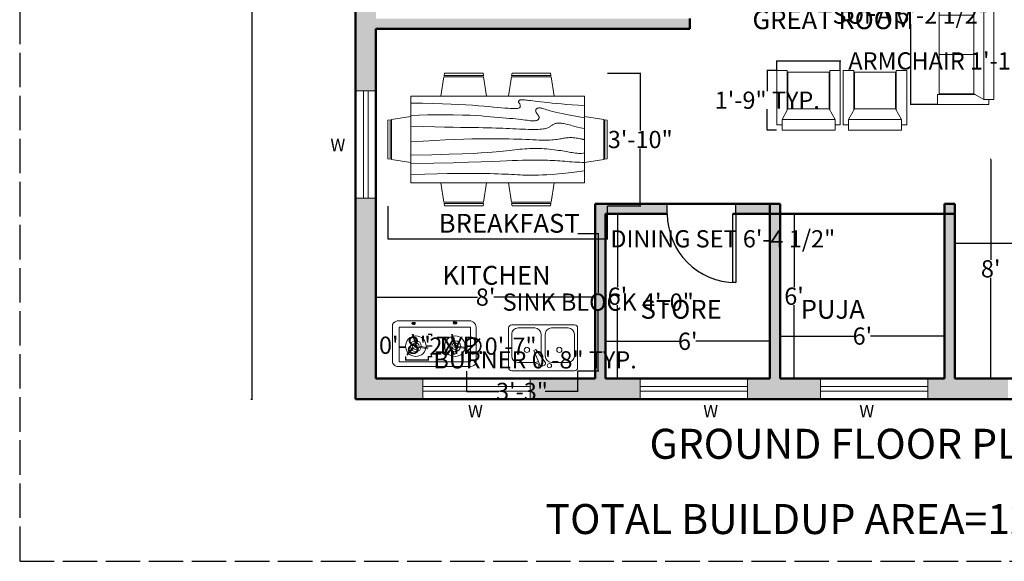
# Model space of a CAD drawing. Units: inches. Extents: x 2905 to 3459, y 4225 to 4672.
# Tile 1 of 3: x 2905 to 3248, y 4225 to 4414. Entities that reach past the tile are written whole.
import ezdxf

# ---------------------------------------------------------------- set-up
doc = ezdxf.new("R2010")
doc.units = ezdxf.units.IN
doc.header["$MEASUREMENT"] = 0
doc.linetypes.add('ACAD_ISO02W100', pattern=[15, 12, -3])
doc.layers.get('0').update_dxf_attribs({"color": 252})
for name, color, linetype, lineweight in [('A-ANNO-DIMS', 2, 'Continuous', 18), ('A-ANNO-TEXT', 7, 'Continuous', 18), ('A-ANNO-TTLB', 7, 'ACAD_ISO02W100', 25), ('A-AREA-IDEN', 7, 'Continuous', 25), ('A-DOOR', 3, 'Continuous', 25), ('A-EQPM', 8, 'Continuous', 18), ('A-FLOR-FIXT', 9, 'Continuous', 18), ('A-GLAZ', 4, 'Continuous', 18), ('A-WALL-PATT', 251, 'Continuous', 13), ('furniture', 8, 'Continuous', 18), ('walls', 251, 'Continuous', 50)]:
    doc.layers.add(name, color=color, linetype=linetype, lineweight=lineweight)
doc.styles.add('ATT', font='TXT')
doc.styles.get("Standard").update_dxf_attribs({"font": 'arial.ttf'})
doc.dimstyles.get("Standard").update_dxf_attribs({"dimtxt": 6, "dimasz": 0.18, "dimexe": 0.18, "dimexo": 0.0625, "dimgap": 0.09, "dimtad": 0, "dimtih": 1, "dimtoh": 1, "dimzin": 0, "dimdsep": 46, "dimlunit": 3, "dimtxsty": 'Standard', "dimcen": 0.09, "dimadec": 0, "dimazin": 0, "dimtfac": 1, "dimtofl": 0, "dimtmove": 0, "dimatfit": 3, "dimfxl": 1, "dimtolj": 1, "dimtzin": 0, "dimarcsym": 0})

# ---------------------------------------------------------------- blocks, each defined once
blk = doc.blocks.new('*U2')
for p, q in [((0, 0), (0, -6)), ((40, 0), (40, -6))]:
    blk.add_line(p, q)
blk.add_lwpolyline([(0, 0), (0, 40), (1.75, 40), (1.75, 0)], close=True)
blk.add_arc((0, 0), 40, 0, 90)
blk = doc.blocks.new('15PSNK10')
at = {"color": 0, "linetype": 'ByBlock'}
for p, q in [((0, 15), (0, -15)), ((20.5, 16.5), (1.5, 16.5)), ((7, 15), (17.5, 15)), ((22, -15), (22, 15)), ((4, 4), (4, 12)), ((20.5, 12), (20.5, 4)), ((2.37, -0.1), (2.77, 0.6)), ((10.18, -3.57), (4.27, 0.87)), ((17.5, 1), (7, 1)), ((2.88, -1.54), (9.68, -4.43)), ((4, -12), (4, -4)), ((7.04, -1), (17.5, -1)), ((9.68, -4.43), (10.18, -3.57)), ((20.5, -4), (20.5, -12)), ((1.5, -16.5), (20.5, -16.5)), ((17.5, -15), (7, -15))]:
    blk.add_line(p, q, dxfattribs=at)
for centre, radius in [((10, 7.75), 1.25), ((2.5, 3), 1), ((2.5, -3), 1), ((10, -7.75), 1.25)]:
    blk.add_circle(centre, radius, dxfattribs=at)
for centre, radius, start, end in [((1.5, 15), 1.5, 90, 180), ((7, 12), 3, 90, 180), ((17.5, 12), 3, 0, 90), ((20.5, 15), 1.5, 0, 90), ((3.63, 0.1), 1, 50.5377, 150), ((7, 4), 3, 180, 270), ((17.5, 4), 3, 270, 0), ((3.23, -0.6), 1, 150, 249.4623), ((7, -4), 3, 146.607, 180), ((17.5, -4), 3, 0, 90), ((7, -12), 3, 180, 270), ((17.5, -12), 3, 270, 0), ((1.5, -15), 1.5, 180, 270), ((20.5, -15), 1.5, 270, 0)]:
    blk.add_arc(centre, radius, start, end, dxfattribs=at)
at = {"color": 0, "linetype": 'ByBlock', "style": 'ATT'}
for tag, p, flags in [('ITEM', (0, -26), 3), ('ROOM_NUMBER', (0, -35), 1)]:
    blk.add_attdef(tag, p, '', height=6, dxfattribs=dict(at, flags=flags))
blk = doc.blocks.new('Dining Set - 36 x 72 in.')
for p, q in [((-22.2343, 26.00059), (-23.4847, 17.99762)), ((-22.2304, 26), (-5.7608, 26)), ((-22, 27.5), (-22.1562, 26.50042)), ((-5.8416, 26.5), (-22.1534, 26.5)), ((-22, 27.5), (-6, 27.5)), ((-5.8437, 26.49966), (-6, 27.5)), ((-4.5152, 17.99762), (-5.7655, 25.99926)), ((5.7657, 26.00059), (4.5153, 17.99762)), ((5.7696, 26), (22.2392, 26)), ((6, 27.5), (5.8438, 26.50042)), ((22.1584, 26.5), (5.8466, 26.5)), ((6, 27.5), (22, 27.5)), ((22.1563, 26.49966), (22, 27.5)), ((23.4848, 17.99762), (22.2345, 25.99926)), ((36, 18), (-36, 18)), ((-36, 18), (-36, -18)), ((36, -18), (36, 18)), ((-44.0006, 8.23428), (-35.9976, 9.48474)), ((-44, 8.23041), (-44, -8.23915)), ((44.0006, 8.23428), (35.9976, 9.48474)), ((44, 8.23041), (44, -8.23915)), ((-45.5, 8), (-44.5004, 8.15617)), ((-45.5, 8), (-45.5, -8)), ((-44.5, -8.15843), (-44.5, 8.15338)), ((44.5, -8.15843), (44.5, 8.15338)), ((45.5, 8), (44.5005, 8.15617)), ((45.5, 8), (45.5, -8)), ((-44.4997, -8.15631), (-45.5, -8)), ((44.4997, -8.15631), (45.5, -8)), ((-35.9976, -9.48476), (-43.9993, -8.2345)), ((35.9976, -9.48476), (43.9993, -8.2345)), ((-36, -18), (36, -18)), ((-22.2343, -26.0006), (-23.4847, -17.99762)), ((-4.5152, -17.99762), (-5.7655, -25.99928)), ((5.7657, -26.0006), (4.5153, -17.99762)), ((23.4848, -17.99762), (22.2345, -25.99928)), ((-22.2304, -26), (-5.7608, -26)), ((-22, -27.5), (-22.1562, -26.50044)), ((-5.8416, -26.5), (-22.1534, -26.5)), ((-22, -27.5), (-6, -27.5)), ((-5.8437, -26.49967), (-6, -27.5)), ((5.7696, -26), (22.2392, -26)), ((6, -27.5), (5.8438, -26.50044)), ((22.1584, -26.5), (5.8466, -26.5)), ((6, -27.5), (22, -27.5)), ((22.1563, -26.49967), (22, -27.5))]:
    blk.add_line(p, q)
for points in [[(-36, 15), (-31.1772, 14.97754), (-26.8079, 14.91406), (-22.8538, 14.81543), (-19.276, 14.6875), (-16.0362, 14.53613), (-13.0957, 14.36718), (-10.4159, 14.18652), (-7.9583, 14), (-5.6904, 13.81315), (-3.6035, 13.63021), (-1.6954, 13.45508), (0.0365, 13.29166), (1.5945, 13.14388), (2.9811, 13.01562), (4.1988, 12.9108), (5.25, 12.83333), (6.1393, 12.78613), (6.8802, 12.76823), (7.4883, 12.77767), (7.9792, 12.8125), (8.3685, 12.87077), (8.6719, 12.95052), (8.9049, 13.0498), (9.0833, 13.16666), (9.2205, 13.29899), (9.3216, 13.44401), (9.3895, 13.59879), (9.4271, 13.76041), (9.4373, 13.92594), (9.4232, 14.09245), (9.3875, 14.257), (9.3333, 14.41666), (9.2638, 14.56917), (9.1836, 14.71484), (9.0975, 14.85465), (9.0104, 14.98958), (8.9272, 15.1206), (8.8529, 15.2487), (8.7922, 15.37483), (8.75, 15.5), (8.7305, 15.62467), (8.7344, 15.74739), (8.7617, 15.86621), (8.8125, 15.97916), (8.8867, 16.08431), (8.9844, 16.17968), (9.1055, 16.26334), (9.25, 16.33333), (9.4189, 16.38802), (9.6172, 16.42708), (9.8506, 16.45052), (10.125, 16.45833), (10.4463, 16.45052), (10.8203, 16.42708), (11.2529, 16.38802), (11.75, 16.33333), (12.3184, 16.26318), (12.9694, 16.17838), (13.7151, 16.07991), (14.5677, 15.96875), (15.5395, 15.84586), (16.6426, 15.71224), (17.8893, 15.56884), (19.2917, 15.41666), (20.859, 15.25667), (22.5879, 15.08984), (24.4721, 14.91715), (26.5052, 14.73958), (28.6809, 14.5581), (30.9929, 14.3737), (33.4347, 14.18733), (36, 14)], [(-36, 10), (-28.9766, 10.14274), (-23.1725, 10.20442), (-18.4241, 10.19775), (-14.5677, 10.13541), (-11.4399, 10.03011), (-8.877, 9.89453), (-6.7154, 9.74137), (-4.7917, 9.58333), (-2.9698, 9.43082), (-1.2246, 9.28515), (0.4415, 9.14534), (2.026, 9.01041), (3.5266, 8.87939), (4.9408, 8.7513), (6.266, 8.62516), (7.5, 8.5), (8.6411, 8.37549), (9.6914, 8.2539), (10.6538, 8.13818), (11.5312, 8.03125), (12.3267, 7.93603), (13.043, 7.85547), (13.6831, 7.79248), (14.25, 7.75), (14.7471, 7.7303), (15.1797, 7.73307), (15.5537, 7.75732), (15.875, 7.80208), (16.1494, 7.86637), (16.3828, 7.94922), (16.5811, 8.04964), (16.75, 8.16666), (16.8944, 8.29915), (17.0143, 8.44531), (17.1089, 8.60319), (17.1771, 8.77083), (17.218, 8.94629), (17.2305, 9.1276), (17.2137, 9.31282), (17.1667, 9.5), (17.0895, 9.6875), (16.987, 9.875), (16.8649, 10.0625), (16.7292, 10.25), (16.5856, 10.4375), (16.4401, 10.625), (16.2985, 10.8125), (16.1667, 11), (16.05, 11.18733), (15.9518, 11.3737), (15.8752, 11.5581), (15.8229, 11.73958), (15.798, 11.91715), (15.8034, 12.08984), (15.842, 12.25667), (15.9167, 12.41666), (16.0295, 12.56836), (16.1784, 12.70833), (16.3605, 12.83268), (16.5729, 12.9375), (16.8127, 13.01888), (17.0768, 13.07291), (17.3625, 13.0957), (17.6667, 13.08333), (17.9894, 13.03312), (18.3418, 12.94726), (18.7382, 12.82918), (19.1927, 12.68229), (19.7195, 12.51001), (20.3327, 12.31575), (21.0465, 12.10294), (21.875, 11.875), (22.8357, 11.63354), (23.959, 11.37304), (25.2786, 11.08618), (26.8282, 10.76562), (28.6414, 10.40405), (30.752, 9.99414), (33.1936, 9.52856), (36, 9)], [(-36, 5.5), (-30.7157, 5.3348), (-26.069, 5.20963), (-21.9946, 5.11767), (-18.4271, 5.05208), (-15.3009, 5.00602), (-12.5508, 4.97265), (-10.1112, 4.94515), (-7.9167, 4.91666), (-5.909, 4.88167), (-4.0586, 4.83984), (-2.3429, 4.79215), (-0.7396, 4.73958), (0.7739, 4.6831), (2.22, 4.6237), (3.6213, 4.56233), (5, 4.5), (6.373, 4.43782), (7.7344, 4.3776), (9.0723, 4.32129), (10.375, 4.27083), (11.6309, 4.22819), (12.8281, 4.19531), (13.9551, 4.17415), (15, 4.16666), (15.954, 4.17448), (16.819, 4.19791), (17.6001, 4.23698), (18.3021, 4.29166), (18.9299, 4.36198), (19.4883, 4.44791), (19.9823, 4.54948), (20.4167, 4.66666), (20.7969, 4.79899), (21.1302, 4.94401), (21.4245, 5.09879), (21.6875, 5.26041), (21.9271, 5.42594), (22.1511, 5.59245), (22.3672, 5.757), (22.5834, 5.91666), (22.8065, 6.06868), (23.0404, 6.21093), (23.2879, 6.34147), (23.5521, 6.45833), (23.8358, 6.55957), (24.142, 6.64323), (24.4735, 6.70735), (24.8334, 6.75), (25.2235, 6.76969), (25.642, 6.76692), (26.0858, 6.74267), (26.5521, 6.69791), (27.0379, 6.63362), (27.5404, 6.55078), (28.0565, 6.45036), (28.5834, 6.33333), (29.1242, 6.19987), (29.7071, 6.04687), (30.3661, 5.87044), (31.1354, 5.66666), (32.0493, 5.43164), (33.142, 5.16146), (34.4475, 4.85221), (36, 4.5)], [(-36, -1), (-30.7915, -0.6591), (-26.0195, -0.38216), (-21.6519, -0.16284), (-17.6563, 0.00521), (-14.0005, 0.12833), (-10.6523, 0.21289), (-7.5796, 0.26522), (-4.75, 0.29166), (-2.134, 0.29793), (0.2878, 0.28711), (2.5317, 0.26163), (4.6146, 0.22396), (6.5529, 0.17651), (8.3633, 0.12174), (10.0623, 0.06209), (11.6667, 0), (13.1899, -0.06201), (14.6341, -0.1211), (15.9982, -0.17432), (17.2813, -0.21875), (18.4823, -0.25147), (19.6003, -0.26953), (20.6343, -0.27002), (21.5834, -0.25), (22.4481, -0.20768), (23.2357, -0.14584), (23.9549, -0.06836), (24.6146, 0.02083), (25.2235, 0.11784), (25.7904, 0.21875), (26.3241, 0.31966), (26.8334, 0.41666), (27.3265, 0.50618), (27.8099, 0.58593), (28.2894, 0.65397), (28.7709, 0.70833), (29.2601, 0.74707), (29.763, 0.76823), (30.2855, 0.76985), (30.8334, 0.75), (31.4088, 0.70784), (31.9994, 0.64713), (32.589, 0.57275), (33.1615, 0.48958), (33.7008, 0.4025), (34.1908, 0.3164), (34.6153, 0.23616), (34.9584, 0.16666), (35.2099, 0.11165), (35.3848, 0.07031), (35.504, 0.04069), (35.5886, 0.02083), (35.6594, 0.00879), (35.7377, 0.0026), (35.8442, 0.00032), (36, 0)], [(-36, -6.5), (-27.1843, -6.31267), (-20.084, -6.1263), (-14.469, -5.9419), (-10.1094, -5.76042), (-6.7752, -5.58285), (-4.2363, -5.41016), (-2.2629, -5.24333), (-0.625, -5.08334), (0.8708, -4.93099), (2.2715, -4.78646), (3.5872, -4.64974), (4.8281, -4.52084), (6.0046, -4.39974), (7.127, -4.28646), (8.2053, -4.18099), (9.25, -4.08334), (10.2705, -3.99382), (11.2734, -3.91407), (12.2647, -3.84603), (13.25, -3.79167), (14.2354, -3.75293), (15.2266, -3.73177), (16.2295, -3.73015), (17.25, -3.75), (18.2912, -3.79248), (19.3451, -3.85547), (20.4009, -3.93604), (21.4479, -4.03125), (22.4754, -4.13819), (23.4727, -4.25391), (24.4289, -4.37549), (25.3334, -4.5), (26.1785, -4.62492), (26.9694, -4.74935), (27.7145, -4.87281), (28.4219, -4.99479), (29.1, -5.11483), (29.7572, -5.23242), (30.4016, -5.34709), (31.0417, -5.45834), (31.6837, -5.56437), (32.3262, -5.65821), (32.9658, -5.73153), (33.599, -5.77604), (34.2224, -5.78345), (34.8327, -5.74545), (35.4264, -5.65373), (36, -5.5)], [(-36, -10), (-26.4022, -9.81299), (-18.4675, -9.62891), (-11.9839, -9.45069), (-6.7396, -9.28125), (-2.5226, -9.12354), (0.8789, -8.98047), (3.6769, -8.85498), (6.0833, -8.75), (8.2767, -8.66765), (10.3021, -8.60677), (12.1712, -8.56543), (13.8958, -8.54167), (15.4876, -8.53353), (16.9583, -8.53907), (18.3197, -8.55632), (19.5834, -8.58334), (20.7616, -8.61841), (21.8685, -8.66081), (22.9188, -8.71004), (23.9271, -8.76563), (24.9081, -8.82707), (25.8763, -8.89388), (26.8465, -8.96558), (27.8334, -9.04167), (28.8474, -9.12118), (29.8828, -9.20117), (30.93, -9.27824), (31.9792, -9.34896), (33.0205, -9.40991), (34.0443, -9.45768), (35.0407, -9.48885), (36, -9.5)], [(-36, -14.5), (-30.0881, -14.33513), (-25.0332, -14.21224), (-20.7312, -14.12647), (-17.0781, -14.07292), (-13.97, -14.04671), (-11.3027, -14.04297), (-8.9724, -14.05681), (-6.875, -14.08334), (-4.9224, -14.11833), (-3.0905, -14.16016), (-1.3709, -14.20785), (0.2448, -14.26042), (1.7647, -14.3169), (3.1973, -14.3763), (4.5507, -14.43767), (5.8333, -14.5), (7.0554, -14.5621), (8.235, -14.62175), (9.3922, -14.67652), (10.5469, -14.72396), (11.7192, -14.76164), (12.929, -14.78711), (14.1965, -14.79794), (15.5417, -14.79167), (16.9933, -14.76424), (18.6152, -14.70508), (20.4804, -14.60197), (22.6615, -14.44271), (25.2312, -14.21509), (28.2624, -13.9069), (31.8277, -13.50594), (36, -13)]]:
    blk.add_lwpolyline(points)
blk = doc.blocks.new('FABRIC SOFA 4S')
at = {"layer": 'furniture'}
for p, q in [((3, 54), (34, 54)), ((3, 51), (3, 54)), ((34, 48), (34, 54)), ((0, -51), (0, 51)), ((6, 51), (0, 51)), ((6, -51), (6, 51)), ((12, 47.63), (6, 51)), ((11.14, 48), (34, 48)), ((33, 23.81), (12, 23.81)), ((33, 0), (12, 0)), ((33, -23.81), (12, -23.81)), ((6, -51), (0, -51)), ((3, -54), (3, -51)), ((6, -51), (12, -47.63)), ((11.54, -48), (34, -48)), ((34, -48), (34, -54)), ((3, -54), (34, -54))]:
    blk.add_line(p, q, dxfattribs=at)
blk.add_lwpolyline([(12, -47.63), (12, 47.63), (33, 47.63), (33, -47.63)], close=True, dxfattribs=at)
blk = doc.blocks.new('FABRIC SOFA 1S')
at = {"layer": 'furniture'}
for p, q in [((3, 18.12), (34, 18.12)), ((3, 15.12), (3, 18.12)), ((34, 12.12), (34, 18.12)), ((0, -15.12), (0, 15.12)), ((6, 15.12), (0, 15.12)), ((6, -15.12), (6, 15.12)), ((12, 11.75), (6, 15.12)), ((11.33, 12.12), (34, 12.12)), ((6, -15.12), (0, -15.12)), ((3, -18.12), (3, -15.12)), ((6, -15.12), (12, -11.75)), ((11.33, -12.12), (34, -12.12)), ((34, -12.12), (34, -18.12)), ((3, -18.12), (34, -18.12))]:
    blk.add_line(p, q, dxfattribs=at)
blk.add_lwpolyline([(12, -11.75), (12, 11.75), (33, 11.75), (33, -11.75)], close=True, dxfattribs=at)
blk = doc.blocks.new('*D17')
at = {"layer": 'A-ANNO-DIMS', "color": 0, "lineweight": -2, "transparency": 16777216}
for p, q in [((3243.15, 4365.3), (3243.03, 4365.3)), ((3243.21, 4365.12), (3243.21, 4330.25)), ((3243.21, 4289.08), (3243.21, 4323.95)), ((3243.03, 4288.9), (3243.39, 4288.9))]:
    blk.add_line(p, q, dxfattribs=at)
at = {"layer": 'A-ANNO-DIMS', "color": 0, "transparency": 16777216}
for points in [[(3243.18, 4365.12), (3243.24, 4365.12), (3243.21, 4365.3)], [(3243.18, 4289.08), (3243.24, 4289.08), (3243.21, 4288.9)]]:
    blk.add_solid(points, dxfattribs=at)
at = {"layer": 'Defpoints', "color": 0, "transparency": 16777216}
for p in [(3243.21, 4365.3), (3243.21, 4365.3), (3242.97, 4288.9)]:
    blk.add_point(p, dxfattribs=at)
at = {"layer": 'A-ANNO-DIMS', "color": 0, "transparency": 16777216, "insert": (3243.21, 4327.1), "char_height": 6, "attachment_point": 5}
blk.add_mtext("\\A1;8'", dxfattribs=at)
blk = doc.blocks.new('*D18')
at = {"layer": 'A-ANNO-DIMS', "color": 0, "lineweight": -2, "transparency": 16777216}
for p, q in [((3230.73, 4336.07), (3230.73, 4336.19)), ((3230.91, 4336.01), (3284.92, 4336.01)), ((3348.73, 4336.01), (3294.72, 4336.01)), ((3348.91, 4336.07), (3348.91, 4336.19))]:
    blk.add_line(p, q, dxfattribs=at)
at = {"layer": 'A-ANNO-DIMS', "color": 0, "transparency": 16777216}
for points in [[(3230.91, 4336.04), (3230.91, 4335.98), (3230.73, 4336.01)], [(3348.73, 4336.04), (3348.73, 4335.98), (3348.91, 4336.01)]]:
    blk.add_solid(points, dxfattribs=at)
at = {"layer": 'Defpoints', "color": 0, "transparency": 16777216}
for p in [(3230.73, 4336.01), (3348.91, 4336.01), (3348.91, 4336.01)]:
    blk.add_point(p, dxfattribs=at)
at = {"layer": 'A-ANNO-DIMS', "color": 0, "transparency": 16777216, "insert": (3289.82, 4336.01), "char_height": 6, "attachment_point": 5}
blk.add_mtext("\\A1;12'", dxfattribs=at)
blk = doc.blocks.new('*D19')
at = {"layer": 'A-ANNO-DIMS', "color": 0, "lineweight": -2, "transparency": 16777216}
for p, q in [((3174.67, 4346.02), (3174.67, 4320.7)), ((3174.73, 4346.2), (3174.85, 4346.2)), ((3174.67, 4289.08), (3174.67, 4314.4)), ((3174.73, 4288.9), (3174.85, 4288.9))]:
    blk.add_line(p, q, dxfattribs=at)
at = {"layer": 'A-ANNO-DIMS', "color": 0, "transparency": 16777216}
for points in [[(3174.64, 4346.02), (3174.7, 4346.02), (3174.67, 4346.2)], [(3174.64, 4289.08), (3174.7, 4289.08), (3174.67, 4288.9)]]:
    blk.add_solid(points, dxfattribs=at)
at = {"layer": 'Defpoints', "color": 0, "transparency": 16777216}
for p in [(3174.67, 4346.2), (3174.67, 4288.9), (3174.67, 4288.9)]:
    blk.add_point(p, dxfattribs=at)
at = {"layer": 'A-ANNO-DIMS', "color": 0, "transparency": 16777216, "insert": (3174.67, 4317.55), "char_height": 6, "attachment_point": 5}
blk.add_mtext("\\A1;6'", dxfattribs=at)
blk = doc.blocks.new('*D20')
at = {"layer": 'A-ANNO-DIMS', "color": 0, "lineweight": -2, "transparency": 16777216}
for p, q in [((3169.85, 4303.75), (3169.85, 4303.86)), ((3170.03, 4303.68), (3195.63, 4303.68)), ((3226.97, 4303.68), (3201.37, 4303.68)), ((3227.15, 4303.75), (3227.15, 4303.86))]:
    blk.add_line(p, q, dxfattribs=at)
at = {"layer": 'A-ANNO-DIMS', "color": 0, "transparency": 16777216}
for points in [[(3170.03, 4303.71), (3170.03, 4303.65), (3169.85, 4303.68)], [(3226.97, 4303.71), (3226.97, 4303.65), (3227.15, 4303.68)]]:
    blk.add_solid(points, dxfattribs=at)
at = {"layer": 'Defpoints', "color": 0, "transparency": 16777216}
for p in [(3169.85, 4303.68), (3227.15, 4303.68), (3227.15, 4303.68)]:
    blk.add_point(p, dxfattribs=at)
at = {"layer": 'A-ANNO-DIMS', "color": 0, "transparency": 16777216, "insert": (3198.5, 4303.68), "char_height": 6, "attachment_point": 5}
blk.add_mtext("\\A1;6'", dxfattribs=at)
blk = doc.blocks.new('*D21')
at = {"layer": 'A-ANNO-DIMS', "color": 0, "lineweight": -2, "transparency": 16777216}
for p, q in [((3113.13, 4346.02), (3113.13, 4320.7)), ((3113.19, 4346.2), (3113.31, 4346.2)), ((3113.13, 4289.08), (3113.13, 4314.4)), ((3113.19, 4288.9), (3113.31, 4288.9))]:
    blk.add_line(p, q, dxfattribs=at)
at = {"layer": 'A-ANNO-DIMS', "color": 0, "transparency": 16777216}
for points in [[(3113.1, 4346.02), (3113.16, 4346.02), (3113.13, 4346.2)], [(3113.1, 4289.08), (3113.16, 4289.08), (3113.13, 4288.9)]]:
    blk.add_solid(points, dxfattribs=at)
at = {"layer": 'Defpoints', "color": 0, "transparency": 16777216}
for p in [(3113.13, 4346.2), (3113.13, 4288.9), (3113.13, 4288.9)]:
    blk.add_point(p, dxfattribs=at)
at = {"layer": 'A-ANNO-DIMS', "color": 0, "transparency": 16777216, "insert": (3113.13, 4317.55), "char_height": 6, "attachment_point": 5}
blk.add_mtext("\\A1;6'", dxfattribs=at)
blk = doc.blocks.new('*D22')
at = {"layer": 'A-ANNO-DIMS', "color": 0, "lineweight": -2, "transparency": 16777216}
for p, q in [((3108.97, 4301.79), (3108.97, 4301.68)), ((3109.15, 4301.86), (3134.75, 4301.86)), ((3166.09, 4301.86), (3140.48, 4301.86)), ((3166.27, 4301.92), (3166.27, 4302.04))]:
    blk.add_line(p, q, dxfattribs=at)
at = {"layer": 'A-ANNO-DIMS', "color": 0, "transparency": 16777216}
for points in [[(3109.15, 4301.89), (3109.15, 4301.83), (3108.97, 4301.86)], [(3166.09, 4301.89), (3166.09, 4301.83), (3166.27, 4301.86)]]:
    blk.add_solid(points, dxfattribs=at)
at = {"layer": 'Defpoints', "color": 0, "transparency": 16777216}
for p in [(3108.97, 4301.86), (3166.27, 4301.86), (3166.27, 4301.86)]:
    blk.add_point(p, dxfattribs=at)
at = {"layer": 'A-ANNO-DIMS', "color": 0, "transparency": 16777216, "insert": (3137.62, 4301.86), "char_height": 6, "attachment_point": 5}
blk.add_mtext("\\A1;6'", dxfattribs=at)
blk = doc.blocks.new('*D24')
at = {"layer": 'A-ANNO-DIMS', "color": 0, "lineweight": -2, "transparency": 16777216}
for p, q in [((3028.98, 4317.18), (3028.98, 4317.07)), ((3029.16, 4317.25), (3064.33, 4317.25)), ((3105.21, 4317.25), (3070.04, 4317.25)), ((3105.39, 4317.18), (3105.39, 4317.07))]:
    blk.add_line(p, q, dxfattribs=at)
at = {"layer": 'A-ANNO-DIMS', "color": 0, "transparency": 16777216}
for points in [[(3029.16, 4317.28), (3029.16, 4317.22), (3028.98, 4317.25)], [(3105.21, 4317.28), (3105.21, 4317.22), (3105.39, 4317.25)]]:
    blk.add_solid(points, dxfattribs=at)
at = {"layer": 'Defpoints', "color": 0, "transparency": 16777216}
for p in [(3028.98, 4317.25), (3105.39, 4317.25), (3105.39, 4317.25)]:
    blk.add_point(p, dxfattribs=at)
at = {"layer": 'A-ANNO-DIMS', "color": 0, "transparency": 16777216, "insert": (3067.19, 4317.25), "char_height": 6, "attachment_point": 5}
blk.add_mtext("\\A1;8'", dxfattribs=at)
blk = doc.blocks.new('*D25')
at = {"layer": 'A-ANNO-DIMS', "color": 0, "lineweight": -2, "transparency": 16777216}
for p, q in [((2985.39, 4615.99), (2985.98, 4615.99)), ((2985.8, 4615.81), (2985.8, 4452.02)), ((2985.8, 4281.92), (2985.8, 4445.71)), ((2985.39, 4281.74), (2985.98, 4281.74))]:
    blk.add_line(p, q, dxfattribs=at)
at = {"layer": 'A-ANNO-DIMS', "color": 0, "transparency": 16777216}
for points in [[(2985.77, 4615.81), (2985.83, 4615.81), (2985.8, 4615.99)], [(2985.77, 4281.92), (2985.83, 4281.92), (2985.8, 4281.74)]]:
    blk.add_solid(points, dxfattribs=at)
at = {"layer": 'Defpoints', "color": 0, "transparency": 16777216}
for p in [(2985.32, 4615.99), (2985.32, 4281.74), (2985.8, 4281.74)]:
    blk.add_point(p, dxfattribs=at)
at = {"layer": 'A-ANNO-DIMS', "color": 0, "transparency": 16777216, "insert": (2985.8, 4448.86), "char_height": 6, "attachment_point": 5}
blk.add_mtext("\\A1;35'", dxfattribs=at)
blk = doc.blocks.new('WIN-PLAN-STANDARD')
for p, q in [((0, 7.16), (0, 0)), ((37.45, 7.16), (0, 7.16)), ((0, 7.16), (0, 4.38)), ((37.45, 0), (37.45, 7.16)), ((0, 4.38), (37.45, 4.38)), ((37.45, 4.38), (37.45, 2.7)), ((0, 2.7), (37.45, 2.7)), ((0, 0), (37.45, 0))]:
    blk.add_line(p, q)
blk = doc.blocks.new('COOKTOP-BURNER')
for p, q in [((3.4, 4.69), (2.36, 7.73)), ((3.74, 4.7), (2.62, 7.81)), ((4.71, 3.58), (7.87, 2.96)), ((2.54, 3.16), (0.4, 0.64)), ((2.72, 2.87), (0.61, 0.45)), ((4.55, 3.29), (7.8, 2.69))]:
    blk.add_line(p, q)
for radius in [3.58, 1.91, 1.12, 0.464]:
    blk.add_circle((3.58, 3.58), radius)
blk = doc.blocks.new('*D32')
at = {"layer": 'A-ANNO-DIMS', "color": 0, "lineweight": -2, "transparency": 16777216}
for p, q in [((3168.67, 4396.25), (3168.67, 4399.69)), ((3168.85, 4399.51), (3190.61, 4399.51)), ((3190.79, 4396.25), (3190.79, 4399.69)), ((3190.79, 4399.51), (3190.97, 4399.51))]:
    blk.add_line(p, q, dxfattribs=at)
at = {"layer": 'A-ANNO-DIMS', "color": 0, "transparency": 16777216}
for points in [[(3168.85, 4399.54), (3168.85, 4399.48), (3168.67, 4399.51)], [(3190.61, 4399.54), (3190.61, 4399.48), (3190.79, 4399.51)]]:
    blk.add_solid(points, dxfattribs=at)
at = {"layer": 'Defpoints', "color": 0, "transparency": 16777216}
for p in [(3190.79, 4399.51), (3168.67, 4396.19), (3190.79, 4396.19)]:
    blk.add_point(p, dxfattribs=at)
at = {"layer": 'A-ANNO-DIMS', "color": 0, "transparency": 16777216, "insert": (3235.37, 4399.51), "char_height": 6, "attachment_point": 5}
blk.add_mtext('\\A1;ARMCHAIR 1\'-10" TYP.', dxfattribs=at)
blk = doc.blocks.new('*D33')
at = {"layer": 'A-ANNO-DIMS', "color": 0, "lineweight": -2, "transparency": 16777216}
for p, q in [((3168.6, 4396.19), (3165.17, 4396.19)), ((3165.35, 4396.01), (3165.35, 4388.97)), ((3165.35, 4375.62), (3165.35, 4382.66)), ((3168.6, 4375.44), (3165.17, 4375.44))]:
    blk.add_line(p, q, dxfattribs=at)
at = {"layer": 'A-ANNO-DIMS', "color": 0, "transparency": 16777216}
for points in [[(3165.32, 4396.01), (3165.38, 4396.01), (3165.35, 4396.19)], [(3165.32, 4375.62), (3165.38, 4375.62), (3165.35, 4375.44)]]:
    blk.add_solid(points, dxfattribs=at)
at = {"layer": 'Defpoints', "color": 0, "transparency": 16777216}
for p in [(3165.35, 4396.19), (3168.67, 4396.19), (3168.67, 4375.44)]:
    blk.add_point(p, dxfattribs=at)
at = {"layer": 'A-ANNO-DIMS', "color": 0, "transparency": 16777216, "insert": (3165.35, 4385.82), "char_height": 6, "attachment_point": 5}
blk.add_mtext('\\A1;1\'-9" TYP.', dxfattribs=at)
blk = doc.blocks.new('*D38')
at = {"layer": 'A-ANNO-DIMS', "color": 0, "lineweight": -2, "transparency": 16777216}
for p, q in [((3039.29, 4296.52), (3039.29, 4295.22)), ((3047.16, 4296.52), (3047.16, 4295.22)), ((3039.47, 4295.4), (3046.98, 4295.4)), ((3047.16, 4295.4), (3047.34, 4295.4))]:
    blk.add_line(p, q, dxfattribs=at)
at = {"layer": 'A-ANNO-DIMS', "color": 0, "transparency": 16777216}
for points in [[(3039.47, 4295.43), (3039.47, 4295.37), (3039.29, 4295.4)], [(3046.98, 4295.43), (3046.98, 4295.37), (3047.16, 4295.4)]]:
    blk.add_solid(points, dxfattribs=at)
at = {"layer": 'Defpoints', "color": 0, "transparency": 16777216}
for p in [(3039.29, 4296.58), (3047.16, 4296.58), (3047.16, 4295.4)]:
    blk.add_point(p, dxfattribs=at)
at = {"layer": 'A-ANNO-DIMS', "color": 0, "transparency": 16777216, "insert": (3084.44, 4295.4), "char_height": 6, "attachment_point": 5}
blk.add_mtext('\\A1;BURNER 0\'-8" TYP.', dxfattribs=at)
blk = doc.blocks.new('*D39')
at = {"layer": 'A-ANNO-DIMS', "color": 0, "lineweight": -2, "transparency": 16777216}
for p, q in [((3047.22, 4304.39), (3048.52, 4304.39)), ((3048.34, 4304.21), (3048.34, 4303.64)), ((3047.22, 4296.58), (3048.52, 4296.58)), ((3048.34, 4296.76), (3048.34, 4297.33))]:
    blk.add_line(p, q, dxfattribs=at)
at = {"layer": 'A-ANNO-DIMS', "color": 0, "transparency": 16777216}
for points in [[(3048.31, 4304.21), (3048.37, 4304.21), (3048.34, 4304.39)], [(3048.31, 4296.76), (3048.37, 4296.76), (3048.34, 4296.58)]]:
    blk.add_solid(points, dxfattribs=at)
at = {"layer": 'Defpoints', "color": 0, "transparency": 16777216}
for p in [(3047.16, 4304.39), (3048.34, 4304.39), (3047.16, 4296.58)]:
    blk.add_point(p, dxfattribs=at)
at = {"layer": 'A-ANNO-DIMS', "color": 0, "transparency": 16777216, "insert": (3048.34, 4300.48), "char_height": 6, "attachment_point": 5}
blk.add_mtext('\\A1;0\'-8" TYP.', dxfattribs=at)
blk = doc.blocks.new('*D40')
at = {"layer": 'A-ANNO-DIMS', "color": 0, "lineweight": -2, "transparency": 16777216}
for p, q in [((3099.32, 4339.45), (3106.62, 4339.45)), ((3106.44, 4339.27), (3106.44, 4318.71)), ((3106.44, 4291.75), (3106.44, 4312.32)), ((3099.32, 4291.57), (3106.62, 4291.57))]:
    blk.add_line(p, q, dxfattribs=at)
at = {"layer": 'A-ANNO-DIMS', "color": 0, "transparency": 16777216}
for points in [[(3106.41, 4339.27), (3106.47, 4339.27), (3106.44, 4339.45)], [(3106.41, 4291.75), (3106.47, 4291.75), (3106.44, 4291.57)]]:
    blk.add_solid(points, dxfattribs=at)
at = {"layer": 'Defpoints', "color": 0, "transparency": 16777216}
for p in [(3099.26, 4339.45), (3106.44, 4339.45), (3099.26, 4291.57)]:
    blk.add_point(p, dxfattribs=at)
at = {"layer": 'A-ANNO-DIMS', "color": 0, "transparency": 16777216, "insert": (3106.44, 4315.51), "char_height": 6, "attachment_point": 5}
blk.add_mtext('\\A1;SINK BLOCK 4\'-0"', dxfattribs=at)
blk = doc.blocks.new('*D41')
at = {"layer": 'A-ANNO-DIMS', "color": 0, "lineweight": -2, "transparency": 16777216}
for p, q in [((3060.5, 4291.51), (3060.5, 4284.21)), ((3099.26, 4291.51), (3099.26, 4284.21)), ((3060.68, 4284.39), (3071.82, 4284.39)), ((3099.08, 4284.39), (3087.94, 4284.39))]:
    blk.add_line(p, q, dxfattribs=at)
at = {"layer": 'A-ANNO-DIMS', "color": 0, "transparency": 16777216}
for points in [[(3060.68, 4284.42), (3060.68, 4284.36), (3060.5, 4284.39)], [(3099.08, 4284.42), (3099.08, 4284.36), (3099.26, 4284.39)]]:
    blk.add_solid(points, dxfattribs=at)
at = {"layer": 'Defpoints', "color": 0, "transparency": 16777216}
for p in [(3060.5, 4291.57), (3099.26, 4291.57), (3099.26, 4284.39)]:
    blk.add_point(p, dxfattribs=at)
at = {"layer": 'A-ANNO-DIMS', "color": 0, "transparency": 16777216, "insert": (3079.88, 4284.39), "char_height": 6, "attachment_point": 5}
blk.add_mtext('\\A1;3\'-3"', dxfattribs=at)
blk = doc.blocks.new('*D42')
at = {"layer": 'A-ANNO-DIMS', "color": 0, "lineweight": -2, "transparency": 16777216}
for p, q in [((3033.11, 4348.97), (3033.11, 4337.37)), ((3109.6, 4348.97), (3109.6, 4337.37)), ((3033.29, 4337.55), (3109.42, 4337.55)), ((3109.6, 4337.55), (3109.78, 4337.55))]:
    blk.add_line(p, q, dxfattribs=at)
at = {"layer": 'A-ANNO-DIMS', "color": 0, "transparency": 16777216}
for points in [[(3033.29, 4337.58), (3033.29, 4337.52), (3033.11, 4337.55)], [(3109.42, 4337.58), (3109.42, 4337.52), (3109.6, 4337.55)]]:
    blk.add_solid(points, dxfattribs=at)
at = {"layer": 'Defpoints', "color": 0, "transparency": 16777216}
for p in [(3033.11, 4349.03), (3109.6, 4349.03), (3109.6, 4337.55)]:
    blk.add_point(p, dxfattribs=at)
at = {"layer": 'A-ANNO-DIMS', "color": 0, "transparency": 16777216, "insert": (3149.84, 4337.55), "char_height": 6, "attachment_point": 5}
blk.add_mtext('\\A1;DINING SET 6\'-4 1/2"', dxfattribs=at)
blk = doc.blocks.new('*D43')
at = {"layer": 'A-ANNO-DIMS', "color": 0, "lineweight": -2, "transparency": 16777216}
for p, q in [((3109.66, 4395.26), (3121.26, 4395.26)), ((3121.08, 4395.08), (3121.08, 4375.3)), ((3121.08, 4349.21), (3121.08, 4368.99)), ((3109.66, 4349.03), (3121.26, 4349.03))]:
    blk.add_line(p, q, dxfattribs=at)
at = {"layer": 'A-ANNO-DIMS', "color": 0, "transparency": 16777216}
for points in [[(3121.05, 4395.08), (3121.11, 4395.08), (3121.08, 4395.26)], [(3121.05, 4349.21), (3121.11, 4349.21), (3121.08, 4349.03)]]:
    blk.add_solid(points, dxfattribs=at)
at = {"layer": 'Defpoints', "color": 0, "transparency": 16777216}
for p in [(3109.6, 4395.26), (3121.08, 4395.26), (3109.6, 4349.03)]:
    blk.add_point(p, dxfattribs=at)
at = {"layer": 'A-ANNO-DIMS', "color": 0, "transparency": 16777216, "insert": (3121.08, 4372.14), "char_height": 6, "attachment_point": 5}
blk.add_mtext('\\A1;3\'-10"', dxfattribs=at)
blk = doc.blocks.new('*D44')
at = {"layer": 'A-ANNO-DIMS', "color": 0, "lineweight": -2, "transparency": 16777216}
for p, q in [((3224.63, 4446.63), (3215.16, 4446.63)), ((3215.34, 4446.45), (3215.34, 4418.67)), ((3215.34, 4384.49), (3215.34, 4412.28)), ((3224.63, 4384.31), (3215.16, 4384.31))]:
    blk.add_line(p, q, dxfattribs=at)
at = {"layer": 'A-ANNO-DIMS', "color": 0, "transparency": 16777216}
for points in [[(3215.31, 4446.45), (3215.37, 4446.45), (3215.34, 4446.63)], [(3215.31, 4384.49), (3215.37, 4384.49), (3215.34, 4384.31)]]:
    blk.add_solid(points, dxfattribs=at)
at = {"layer": 'Defpoints', "color": 0, "transparency": 16777216}
for p in [(3224.69, 4446.63), (3215.34, 4384.31), (3224.69, 4384.31)]:
    blk.add_point(p, dxfattribs=at)
at = {"layer": 'A-ANNO-DIMS', "color": 0, "transparency": 16777216, "insert": (3215.34, 4415.47), "char_height": 6, "attachment_point": 5}
blk.add_mtext('\\A1;SOFA 5\'-2 1/2"', dxfattribs=at)
blk = doc.blocks.new('*D46')
at = {"layer": 'A-ANNO-DIMS', "color": 0, "lineweight": -2, "transparency": 16777216}
for p, q in [((3042.78, 4300.16), (3042.96, 4300.16)), ((3042.87, 4300.07), (3042.87, 4300.25)), ((3048.61, 4300.16), (3046.64, 4300.16))]:
    blk.add_line(p, q, dxfattribs=at)
at = {"layer": 'A-ANNO-DIMS', "color": 0, "transparency": 16777216}
blk.add_solid([(3046.64, 4300.19), (3046.64, 4300.13), (3046.46, 4300.16)], dxfattribs=at)
at = {"layer": 'Defpoints', "color": 0, "transparency": 16777216}
for p in [(3039.29, 4300.16), (3046.46, 4300.16)]:
    blk.add_point(p, dxfattribs=at)
at = {"layer": 'A-ANNO-DIMS', "color": 0, "transparency": 16777216, "insert": (3066.28, 4300.16), "char_height": 6, "attachment_point": 5}
blk.add_mtext('\\A1;2X ∅0\'-7"', dxfattribs=at)

msp = doc.modelspace()

# ---------------------------------------------------------------- hatches: boundary and pattern name
at = {"layer": 'A-WALL-PATT'}
h = msp.add_hatch(color=256, dxfattribs=at)
h.dxf.hatch_style = 1
h.paths.add_polyline_path([(3291.611, 4382.367), (3288.03, 4382.367), (3288.03, 4349.781), (3348.911, 4349.781), (3348.911, 4353.362), (3291.611, 4353.362)])
h.paths.add_polyline_path([(3291.611, 4410.662), (3288.03, 4410.662), (3288.03, 4405.956), (3291.611, 4405.956)])
h.paths.add_polyline_path([(3356.074, 4439.171), (3348.911, 4439.171), (3348.911, 4387.379), (3356.074, 4387.379)])
h.paths.add_polyline_path([(3356.074, 4366.687), (3348.911, 4366.687), (3348.911, 4288.899), (3341.991, 4288.899), (3341.991, 4286.512), (3341.991, 4281.737), (3356.074, 4281.737)])
h.paths.add_polyline_path([(3310.157, 4286.512, -0.0187698), (3310.247, 4288.899), (3286.75, 4288.899), (3286.75, 4281.737), (3310.157, 4281.737)])
h.paths.add_polyline_path([(3249.298, 4288.899), (3230.73, 4288.899), (3230.73, 4346.199), (3227.148, 4346.199), (3227.148, 4288.899), (3221.363, 4288.899), (3221.363, 4281.737), (3249.298, 4281.737)])
h.paths.add_polyline_path([(3230.73, 4349.781), (3227.148, 4349.781), (3227.148, 4346.199), (3230.73, 4346.199)])
h.paths.add_polyline_path([(3183.911, 4288.899), (3169.848, 4288.899), (3169.848, 4346.199), (3166.267, 4346.199), (3166.267, 4288.899), (3158.463, 4288.899), (3158.463, 4281.737), (3183.911, 4281.737)])
h.paths.add_polyline_path([(3169.848, 4349.781), (3166.267, 4349.781), (3166.267, 4346.199), (3169.848, 4346.199)])
h.paths.add_polyline_path([(3166.267, 4349.781), (3154.383, 4349.781), (3154.383, 4346.199), (3166.267, 4346.199)])
h.paths.add_polyline_path([(3130.507, 4349.781), (3105.385, 4349.781), (3105.385, 4288.899), (3082.76, 4288.899), (3082.76, 4281.737), (3121.011, 4281.737), (3121.011, 4288.899), (3108.967, 4288.899), (3108.967, 4346.199), (3130.507, 4346.199)])
h.paths.add_polyline_path([(3045.307, 4288.899), (3028.985, 4288.899), (3028.985, 4351.673), (3021.822, 4351.673), (3021.822, 4281.737), (3045.307, 4281.737)])
h.paths.add_polyline_path([(3028.985, 4428.302), (3021.822, 4428.302), (3021.822, 4389.126), (3028.985, 4389.126), (3028.985, 4410.662), (3138.383, 4410.662), (3138.383, 4414.244), (3028.985, 4414.244)])
h.paths.add_polyline_path([(3356.074, 4615.988), (3308.212, 4615.988), (3308.212, 4608.826), (3348.911, 4608.826), (3348.911, 4459.863), (3356.074, 4459.863)])
h.paths.add_polyline_path([(3053.98, 4501.489), (3061.351, 4501.489), (3061.351, 4511.329), (3053.98, 4511.329)], flags=9)
h.paths.add_polyline_path([(3141.419, 4592.43), (3152.5, 4592.43), (3152.5, 4602.27), (3141.419, 4602.27)], flags=9)
h.paths.add_polyline_path([(3089.982, 4547.099), (3101.063, 4547.099), (3101.063, 4556.939), (3089.982, 4556.939)], flags=9)
h.paths.add_polyline_path([(3268.583, 4592.669), (3287.963, 4592.669), (3287.963, 4602.509), (3268.583, 4602.509)], flags=9)
h.paths.add_polyline_path([(3307.047, 4423.398), (3314.418, 4423.398), (3314.418, 4433.237), (3307.047, 4433.237)], flags=9)
h.paths.add_polyline_path([(3288.865, 4462.697), (3316.591, 4462.697), (3316.591, 4472.539), (3288.865, 4472.539)], flags=9)
h.paths.add_polyline_path([(3037.676, 4519.097), (3065.402, 4519.097), (3065.402, 4528.939), (3037.676, 4528.939)], flags=9)
h.paths.add_polyline_path([(3265.13, 4583.219), (3291.666, 4583.219), (3291.666, 4593.397), (3265.13, 4593.397)], flags=9)
h.paths.add_polyline_path([(3257.487, 4572.872), (3308.243, 4572.872), (3308.243, 4583.057), (3257.487, 4583.057)], flags=9)
h.paths.add_polyline_path([(3132.382, 4572.872), (3183.138, 4572.872), (3183.138, 4583.057), (3132.382, 4583.057)], flags=9)
h.paths.add_polyline_path([(3134.197, 4582.452), (3175.785, 4582.452), (3175.785, 4592.629), (3134.197, 4592.629)], flags=9)

# ---------------------------------------------------------------- linework, layer by layer
at = {"layer": 'A-ANNO-TTLB'}
for p, q in [((2904.821, 4672.373), (2904.821, 4225.241)), ((2904.821, 4225.241), (3458.552, 4225.241))]:
    msp.add_line(p, q, dxfattribs=at)
at = {"layer": 'A-EQPM'}
for p, q in [((3034.786, 4294.376), (3034.786, 4307.694)), ((3061.068, 4308.983), (3037.029, 4308.983)), ((3061.926, 4306.789), (3037.029, 4306.789)), ((3037.029, 4306.789), (3037.029, 4294.749)), ((3061.926, 4294.749), (3061.926, 4306.789)), ((3063.887, 4294.308), (3063.887, 4306.789)), ((3037.029, 4294.749), (3061.926, 4294.749)), ((3061.926, 4293.023), (3037.029, 4293.023))]:
    msp.add_line(p, q, dxfattribs=at)
for centre, radius, start, end in [((3036.796, 4306.793), 2.203, 83.93636, 156.89401), ((3061.497, 4306.625), 2.396, 3.92707, 100.30452), ((3036.823, 4295.216), 2.203, 202.40616, 275.36382), ((3061.761, 4295.413), 2.396, 273.92707, 332.5308)]:
    msp.add_arc(centre, radius, start, end, dxfattribs=at)
for centre, major_axis, ratio in [((3042.093, 4308.206), (0.653, -0.019), 0.3769734), ((3042.086, 4307.959), (0.608, -0.039), 0.4928397), ((3056.542, 4308.414), (0.653, -0.019), 0.3769734), ((3056.535, 4308.167), (0.608, -0.039), 0.4928397)]:
    msp.add_ellipse(centre, major_axis=major_axis, ratio=ratio, dxfattribs=at)
at = {"layer": 'walls'}
for p, q in [((3021.822, 4281.737), (3021.822, 4615.988)), ((3138.383, 4414.244), (3138.383, 4410.662)), ((3028.985, 4288.899), (3028.985, 4410.662)), ((3028.985, 4410.662), (3138.383, 4410.662)), ((3105.385, 4288.899), (3105.385, 4349.781)), ((3169.848, 4349.781), (3105.385, 4349.781)), ((3166.267, 4288.899), (3166.267, 4349.781)), ((3169.848, 4288.899), (3169.848, 4349.781)), ((3227.148, 4288.899), (3227.148, 4349.781)), ((3230.73, 4349.781), (3227.148, 4349.781)), ((3230.73, 4288.899), (3230.73, 4349.781)), ((3108.967, 4288.899), (3108.967, 4346.199)), ((3130.507, 4346.199), (3108.967, 4346.199)), ((3230.73, 4346.199), (3153.338, 4346.199)), ((3105.385, 4288.899), (3028.985, 4288.899)), ((3166.267, 4288.899), (3108.967, 4288.899)), ((3227.148, 4288.899), (3169.848, 4288.899)), ((3310.247, 4288.899), (3230.73, 4288.899)), ((3356.074, 4281.737), (3021.822, 4281.737))]:
    msp.add_line(p, q, dxfattribs=at)

# ---------------------------------------------------------------- block references
at = {"layer": 'A-DOOR', "xscale": 0.5968803451172152, "yscale": 0.5968803451172152, "zscale": 0.5968803451172152, "rotation": 180}
msp.add_blockref('*U2', (3154.383, 4346.199), dxfattribs=at)
at = {"layer": 'A-EQPM'}
for p in [(3039.29, 4296.579), (3052.954, 4296.579)]:
    msp.add_blockref('COOKTOP-BURNER', p, dxfattribs=at)
at = {"layer": 'A-FLOR-FIXT', "xscale": -0.7283582777072409, "yscale": 0.7283582777072409, "zscale": 0.7283582777072409, "rotation": 270}
msp.add_blockref('15PSNK10', (3087.242, 4291.57), dxfattribs=at)
at = {"layer": 'A-GLAZ', "rotation": 89.99999999999758}
msp.add_blockref('WIN-PLAN-STANDARD', (3028.984, 4351.673), dxfattribs=at)
at = {"layer": 'A-GLAZ'}
for p in [(3045.307, 4281.737), (3121.011, 4281.737), (3183.91, 4281.737)]:
    msp.add_blockref('WIN-PLAN-STANDARD', p, dxfattribs=at)
at = {"layer": 'furniture'}
for name, p, xscale, yscale, zscale, rotation in [('FABRIC SOFA 4S', (3244.312, 4415.471), 0.5770400048926188, 0.5770400048926188, 0.5770400048926188, 180), ('FABRIC SOFA 1S', (3179.728, 4375.441), -0.6103067503488249, 0.6103067503488249, 0.6103067503488249, 270), ('FABRIC SOFA 1S', (3202.892, 4375.441), -0.6103067503488249, 0.6103067503488249, 0.6103067503488249, 270)]:
    msp.add_blockref(name, p, dxfattribs=dict(at, xscale=xscale, yscale=yscale, zscale=zscale, rotation=rotation))
at = {"layer": 'furniture', "xscale": 0.8405729347224816, "yscale": 0.8405729347224816, "zscale": 0.8405729347224816}
msp.add_blockref('Dining Set - 36 x 72 in.', (3071.355, 4372.144), dxfattribs=at)

# ---------------------------------------------------------------- texts
at = {"layer": 'A-ANNO-TEXT'}
for s, height, p in [('W', 4.319, (3013.108, 4368.065)), ('W', 4.319, (3061.057, 4275.374)), ('W', 4.319, (3143.054, 4275.374)), ('W', 4.319, (3197.429, 4275.374)), ('GROUND FLOOR PLAN', 10.45739, (3124.308, 4260.929)), ('TOTAL BUILDUP AREA=1225SQ FT', 10.45739, (3088.083, 4234.734))]:
    msp.add_text(s, height=height, dxfattribs=at).set_placement(p)
at = {"layer": 'A-AREA-IDEN'}
for s, p in [('GREAT ROOM', (3160.193, 4410.561)), ('BREAKFAST', (3050.852, 4339.674)), ('KITCHEN', (3052.128, 4321.549)), ('STORE', (3121.184, 4309.72)), ('PUJA', (3176.996, 4309.72))]:
    msp.add_text(s, height=6.5613, dxfattribs=at).set_placement(p)

# ---------------------------------------------------------------- dimensions: what is measured, and where the dimension line sits
at = {"layer": 'A-ANNO-DIMS'}
for base, p1, p2, angle, text, override, picture, middle in [((2985.804, 4281.737), (2985.324, 4615.988), (2985.324, 4281.737), 90, "35'", {"dimclrd": 0, "dimclre": 0, "dimclrt": 0}, '*D25', (2985.804, 4448.862)), ((3215.345, 4384.311), (3224.693, 4446.631), (3224.693, 4384.311), 270, 'SOFA <>', {"dimdec": 1, "dimlfac": 1, "dimrnd": 0, "dimzin": 1, "dimdsep": 46, "dimlunit": 4, "dimfrac": 2}, '*D44', (3215.345, 4415.471)), ((3165.348, 4396.1914), (3168.6665, 4375.4409), (3168.6665, 4396.1914), 90, '<> TYP.', {"dimdec": 1, "dimlfac": 1, "dimrnd": 0, "dimzin": 1, "dimdsep": 46, "dimlunit": 4, "dimfrac": 2}, '*D33', (3165.348, 4385.8161)), ((3243.207, 4365.299), (3242.966, 4288.899), (3243.208, 4365.299), 90, "8'", {"dimclrd": 0, "dimclre": 0, "dimclrt": 0}, '*D17', (3243.207, 4327.099)), ((3113.125, 4288.899), (3113.125, 4346.199), (3113.125, 4288.899), 90, "6'", {"dimclrd": 0, "dimclre": 0, "dimclrt": 0}, '*D21', (3113.125, 4317.549)), ((3174.668, 4288.899), (3174.668, 4346.199), (3174.668, 4288.899), 90, "6'", {"dimclrd": 0, "dimclre": 0, "dimclrt": 0}, '*D19', (3174.668, 4317.549)), ((3106.442, 4339.451), (3099.259, 4291.57), (3099.259, 4339.451), 90, 'SINK BLOCK <>', {"dimdec": 1, "dimlfac": 1, "dimrnd": 0, "dimzin": 1, "dimdsep": 46, "dimlunit": 4, "dimfrac": 2}, '*D40', (3106.442, 4315.511)), ((3048.339, 4304.391), (3047.158, 4296.579), (3047.158, 4304.391), 90, '<> TYP.', {"dimdec": 1, "dimlfac": 1, "dimrnd": 0, "dimzin": 1, "dimdsep": 46, "dimlunit": 4, "dimfrac": 2}, '*D39', (3048.339, 4300.485))]:
    dim = msp.add_linear_dim(base=base, p1=p1, p2=p2, angle=angle, text=text, dimstyle='Standard', override=override, dxfattribs=at)
    dim.commit()
    dim.dimension.update_dxf_attribs({"geometry": picture, "text_midpoint": middle})
for base, p1, p2, text, override, picture, middle in [((3190.79, 4399.51), (3168.667, 4396.191), (3190.79, 4396.191), 'ARMCHAIR <> TYP.', {"dimdec": 1, "dimlfac": 1, "dimrnd": 0, "dimzin": 1, "dimdsep": 46, "dimlunit": 4, "dimfrac": 2}, '*D32', (3235.368, 4399.51)), ((3109.601, 4337.554), (3033.109, 4349.028), (3109.601, 4349.028), 'DINING SET <>', {"dimdec": 1, "dimlfac": 1, "dimrnd": 0, "dimzin": 1, "dimdsep": 46, "dimlunit": 4, "dimfrac": 2}, '*D42', (3149.835, 4337.554)), ((3348.911, 4336.01), (3230.73, 4336.01), (3348.911, 4336.01), "12'", {"dimclrd": 0, "dimclre": 0, "dimclrt": 0}, '*D18', (3289.821, 4336.01)), ((3105.385, 4317.247), (3028.985, 4317.247), (3105.385, 4317.247), "8'", {"dimclrd": 0, "dimclre": 0, "dimclrt": 0}, '*D24', (3067.185, 4317.247)), ((3047.158, 4295.398), (3039.29, 4296.579), (3047.158, 4296.579), 'BURNER <> TYP.', {"dimdec": 1, "dimlfac": 1, "dimrnd": 0, "dimzin": 1, "dimdsep": 46, "dimlunit": 4, "dimfrac": 2}, '*D38', (3084.443, 4295.398)), ((3227.148, 4303.684), (3169.848, 4303.684), (3227.148, 4303.684), "6'", {"dimclrd": 0, "dimclre": 0, "dimclrt": 0}, '*D20', (3198.498, 4303.684)), ((3166.267, 4301.856), (3108.967, 4301.856), (3166.267, 4301.856), "6'", {"dimclrd": 0, "dimclre": 0, "dimclrt": 0}, '*D22', (3137.617, 4301.856))]:
    dim = msp.add_linear_dim(base=base, p1=p1, p2=p2, text=text, dimstyle='Standard', override=override, dxfattribs=at)
    dim.commit()
    dim.dimension.update_dxf_attribs({"geometry": picture, "text_midpoint": middle})
dim = msp.add_linear_dim(base=(3121.075, 4395.26), p1=(3109.601, 4349.028), p2=(3109.601, 4395.26), angle=90, dimstyle='Standard', override={"dimdec": 1, "dimlfac": 1, "dimrnd": 0, "dimzin": 1, "dimdsep": 46, "dimlunit": 4, "dimfrac": 2}, dxfattribs=at)
dim.commit()
dim.dimension.update_dxf_attribs({"geometry": '*D43', "text_midpoint": (3121.075, 4372.144)})
dim = msp.add_diameter_dim_2p(p1=(3039.29, 4300.163), p2=(3046.459, 4300.163), text='2X <>', dimstyle='Standard', override={"dimdec": 1, "dimlfac": 1, "dimrnd": 0, "dimzin": 1, "dimdsep": 46, "dimlunit": 4, "dimfrac": 2}, dxfattribs=at)
dim.commit()
dim.dimension.update_dxf_attribs({"geometry": '*D46', "text_midpoint": (3048.609, 4300.163), "dimtype": 163})
dim = msp.add_linear_dim(base=(3099.259, 4284.388), p1=(3060.502, 4291.57), p2=(3099.259, 4291.57), dimstyle='Standard', override={"dimdec": 1, "dimlfac": 1, "dimrnd": 0, "dimzin": 1, "dimdsep": 46, "dimlunit": 4, "dimfrac": 2}, dxfattribs=at)
dim.commit()
dim.dimension.update_dxf_attribs({"geometry": '*D41', "text_midpoint": (3079.881, 4284.388)})

doc.saveas('drawing.dxf')
